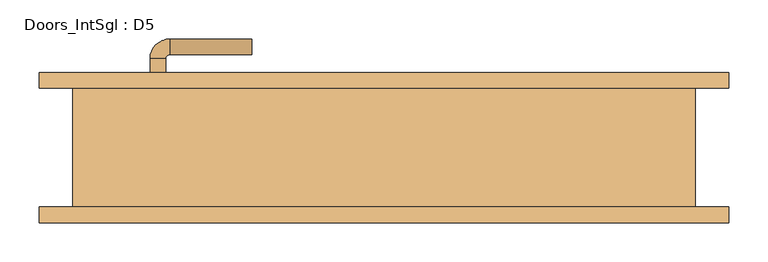
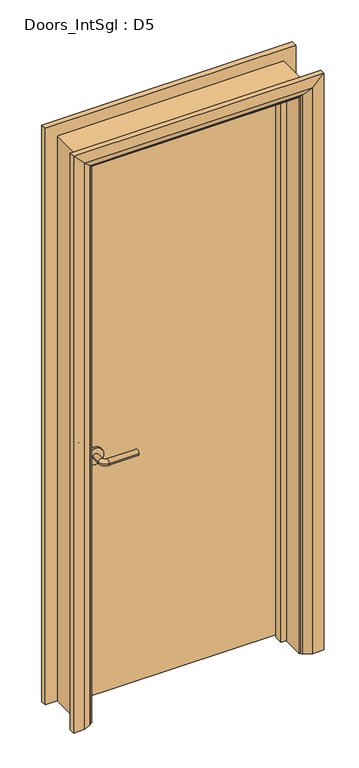
"""IFC4 building model written with IfcOpenShell, lengths in millimetres: door geometry, Doors_IntSgl : D5."""

from ifc_helpers import new_model, si_unit, point, frame, frame_2d, origin, place, context, project, spatial, polyline, circle_curve, ellipse_curve, trimmed, segment, composite_curve, outline, extrude, faceted_brep, source, transform, mapped, element, save
from ifc_brep_helpers import plane_surface, cylinder_surface, revolved_surface, advanced_brep


def doors_intsgl_d5_996c1a6b(model_context):
    return source(origin(), model_context, "Body", "SolidModel", [
        advanced_brep(
        [(-299.4508, 30.2, 900.0), (-279.4508, 30.2, 900.0), (-279.4508, 0.2, 900.0), (-299.4508, 0.2, 900.0), (-274.4508, -4.8, 900.0), (-274.4508, -24.8, 900.0), (-169.4508, -24.8, 900.0), (-169.4508, -4.8, 900.0)],
        [
            (0, 1, circle_curve(frame((-289.4508, 30.2, 900.0), z_axis=(0.0, 1.0, 0.0), x_axis=(1.0, 0.0, 0.0)), 10.0)),
            (1, 0, circle_curve(frame((-289.4508, 30.2, 900.0), z_axis=(0.0, 1.0, 0.0), x_axis=(1.0, 0.0, 0.0)), 10.0)),
            (1, 2),
            (2, 3, circle_curve(frame((-289.4508, 0.2, 900.0), z_axis=(0.0, 1.0, 0.0), x_axis=(1.0, 0.0, 0.0)), 10.0)),
            (3, 0),
            (3, 2, circle_curve(frame((-289.4508, 0.2, 900.0), z_axis=(0.0, 1.0, 0.0), x_axis=(1.0, 0.0, 0.0)), 10.0)),
            (4, 5, circle_curve(frame((-274.4508, -14.8, 900.0), z_axis=(-1.0, 0.0, 0.0), x_axis=(0.0, 1.0, 0.0)), 10.0)),
            (5, 3, circle_curve(frame((-274.4508, 0.2, 900.0), z_axis=(0.0, 0.0, -1.0), x_axis=(-1.0, 0.0, 0.0)), 25.0)),
            (2, 4, circle_curve(frame((-274.4508, 0.2, 900.0), z_axis=(0.0, 0.0, 1.0), x_axis=(-1.0, 0.0, 0.0)), 5.0)),
            (5, 4, circle_curve(frame((-274.4508, -14.8, 900.0), z_axis=(-1.0, 0.0, 0.0), x_axis=(0.0, 1.0, 0.0)), 10.0)),
            (6, 7, circle_curve(frame((-169.4508, -14.8, 900.0), z_axis=(1.0, 0.0, 0.0), x_axis=(0.0, 1.0, 0.0)), 10.0)),
            (7, 6, circle_curve(frame((-169.4508, -14.8, 900.0), z_axis=(1.0, 0.0, 0.0), x_axis=(0.0, 1.0, 0.0)), 10.0)),
            (4, 7),
            (6, 5),
        ],
        [
            plane_surface(frame((-289.4508, 30.2, 900.0), z_axis=(0.0, 1.0, 0.0), x_axis=(0.0, 0.0, 1.0))),
            cylinder_surface(frame((-289.4508, 30.2, 900.0), z_axis=(0.0, 1.0, 0.0), x_axis=(1.0, 0.0, 0.0)), 10.0),
            revolved_surface(trimmed(ellipse_curve(frame((-289.4508, 0.2, 900.0), z_axis=(0.0, -1.0, 0.0), x_axis=(1.0, 0.0, 0.0)), 10.0, 10.0), [point((-299.4508, 0.2, 900.0))], [point((-279.4508, 0.2, 900.0))], True, "CARTESIAN"), (-274.4508, 0.2, 900.0), (0.0, 0.0, -1.0)),
            revolved_surface(trimmed(ellipse_curve(frame((-289.4508, 0.2, 900.0), z_axis=(0.0, -1.0, 0.0), x_axis=(1.0, 0.0, 0.0)), 10.0, 10.0), [point((-279.4508, 0.2, 900.0))], [point((-299.4508, 0.2, 900.0))], True, "CARTESIAN"), (-274.4508, 0.2, 900.0), (0.0, 0.0, -1.0)),
            plane_surface(frame((-169.4508, -14.8, 900.0), z_axis=(1.0, 0.0, 0.0), x_axis=(0.0, 0.0, 1.0))),
            cylinder_surface(frame((-274.4508, -14.8, 900.0), z_axis=(-1.0, 0.0, 0.0), x_axis=(0.0, 1.0, 0.0)), 10.0),
        ],
        [
            (0, [[1, 2]]),
            (1, [[3, 4, 5, -2]]),
            (1, [[-5, 6, -3, -1]]),
            (2, [[7, 8, -4, 9]]),
            (3, [[10, -9, -6, -8]]),
            (4, [[11, 12]]),
            (5, [[13, -11, 14, -7]]),
            (5, [[-14, -12, -13, -10]]),
        ],
    ),
        extrude(outline(composite_curve([segment(trimmed(circle_curve(frame_2d((900.0, -291.9508)), 30.0), [point((900.0, -321.9508))], [point((900.0, -261.9508))], False, "CARTESIAN"), True, "CONTINUOUS"), segment(trimmed(circle_curve(frame_2d((900.0, -291.9508)), 30.0), [point((900.0, -261.9508))], [point((900.0, -321.9508))], False, "CARTESIAN"), True, "CONTINUOUS")], self_intersect=False)), frame((0.0, 30.2, 0.0), z_axis=(0.0, 1.0, 0.0), x_axis=(0.0, 0.0, 1.0)), (0.0, 0.0, 1.0), 8.0),
        advanced_brep(
        [(-299.4508, 84.2, 900.0), (-279.4508, 84.2, 900.0), (-299.4508, 114.2, 900.0), (-279.4508, 114.2, 900.0), (-274.4508, 119.2, 900.0), (-274.4508, 139.2, 900.0), (-169.4508, 139.2, 900.0), (-169.4508, 119.2, 900.0)],
        [
            (0, 1, circle_curve(frame((-289.4508, 84.2, 900.0), z_axis=(0.0, -1.0, 0.0), x_axis=(1.0, 0.0, 0.0)), 10.0)),
            (1, 0, circle_curve(frame((-289.4508, 84.2, 900.0), z_axis=(0.0, -1.0, 0.0), x_axis=(1.0, 0.0, 0.0)), 10.0)),
            (0, 2),
            (2, 3, circle_curve(frame((-289.4508, 114.2, 900.0), z_axis=(0.0, -1.0, 0.0), x_axis=(1.0, 0.0, 0.0)), 10.0)),
            (3, 1),
            (3, 2, circle_curve(frame((-289.4508, 114.2, 900.0), z_axis=(0.0, -1.0, 0.0), x_axis=(1.0, 0.0, 0.0)), 10.0)),
            (4, 3, circle_curve(frame((-274.4508, 114.2, 900.0), z_axis=(0.0, 0.0, 1.0), x_axis=(-1.0, 0.0, 0.0)), 5.0)),
            (2, 5, circle_curve(frame((-274.4508, 114.2, 900.0), z_axis=(0.0, 0.0, -1.0), x_axis=(-1.0, 0.0, 0.0)), 25.0)),
            (5, 4, circle_curve(frame((-274.4508, 129.2, 900.0), z_axis=(-1.0, 0.0, 0.0), x_axis=(0.0, -1.0, 0.0)), 10.0)),
            (4, 5, circle_curve(frame((-274.4508, 129.2, 900.0), z_axis=(-1.0, 0.0, 0.0), x_axis=(0.0, -1.0, 0.0)), 10.0)),
            (6, 7, circle_curve(frame((-169.4508, 129.2, 900.0), z_axis=(1.0, 0.0, 0.0), x_axis=(0.0, -1.0, 0.0)), 10.0)),
            (7, 6, circle_curve(frame((-169.4508, 129.2, 900.0), z_axis=(1.0, 0.0, 0.0), x_axis=(0.0, -1.0, 0.0)), 10.0)),
            (5, 6),
            (7, 4),
        ],
        [
            plane_surface(frame((-289.4508, 84.2, 900.0), z_axis=(0.0, -1.0, 0.0), x_axis=(0.0, 0.0, 1.0))),
            cylinder_surface(frame((-289.4508, 84.2, 900.0), z_axis=(0.0, -1.0, 0.0), x_axis=(1.0, 0.0, 0.0)), 10.0),
            revolved_surface(trimmed(ellipse_curve(frame((-289.4508, 114.2, 900.0), z_axis=(0.0, -1.0, 0.0), x_axis=(1.0, 0.0, 0.0)), 10.0, 10.0), [point((-299.4508, 114.2, 900.0))], [point((-279.4508, 114.2, 900.0))], True, "CARTESIAN"), (-274.4508, 114.2, 900.0), (0.0, 0.0, -1.0)),
            revolved_surface(trimmed(ellipse_curve(frame((-289.4508, 114.2, 900.0), z_axis=(0.0, -1.0, 0.0), x_axis=(1.0, 0.0, 0.0)), 10.0, 10.0), [point((-279.4508, 114.2, 900.0))], [point((-299.4508, 114.2, 900.0))], True, "CARTESIAN"), (-274.4508, 114.2, 900.0), (0.0, 0.0, -1.0)),
            plane_surface(frame((-169.4508, 129.2, 900.0), z_axis=(1.0, 0.0, 0.0), x_axis=(0.0, 0.0, 1.0))),
            cylinder_surface(frame((-274.4508, 129.2, 900.0), z_axis=(-1.0, 0.0, 0.0), x_axis=(0.0, -1.0, 0.0)), 10.0),
        ],
        [
            (0, [[1, 2]]),
            (1, [[-1, 3, 4, 5]]),
            (1, [[-2, -5, 6, -3]]),
            (2, [[7, -4, 8, 9]]),
            (3, [[-8, -6, -7, 10]]),
            (4, [[11, 12]]),
            (5, [[-9, 13, -12, 14]]),
            (5, [[-10, -14, -11, -13]]),
        ],
    ),
        extrude(outline(composite_curve([segment(trimmed(circle_curve(frame_2d((900.0, -291.9508)), 30.0), [point((900.0, -321.9508))], [point((900.0, -261.9508))], False, "CARTESIAN"), True, "CONTINUOUS"), segment(trimmed(circle_curve(frame_2d((900.0, -291.9508)), 30.0), [point((900.0, -261.9508))], [point((900.0, -321.9508))], False, "CARTESIAN"), True, "CONTINUOUS")], self_intersect=False)), frame((0.0, 76.2, 0.0), z_axis=(0.0, 1.0, 0.0), x_axis=(0.0, 0.0, 1.0)), (0.0, 0.0, 1.0), 8.0),
        extrude(outline(polyline([(364.4508, 38.2), (-364.4508, 38.2), (-364.4508, 76.2), (364.4508, 76.2), (364.4508, 38.2)])), frame((0.0, 0.0, 8.0), z_axis=(0.0, 0.0, 1.0), x_axis=(1.0, 0.0, 0.0)), (0.0, 0.0, 1.0), 2060.0),
        advanced_brep(
        [(441.4508, 96.2, 0.0), (441.4508, 76.2, 0.0), (371.4508, 76.2, 0.0), (375.4508, 82.2, 0.0), (401.4508, 96.2, 0.0), (441.4508, 96.2, 2145.0), (441.4508, 76.2, 2145.0), (-441.4508, 76.2, 2145.0), (-441.4508, 76.2, 0.0), (-371.4508, 76.2, 0.0), (-371.4508, 76.2, 2075.0), (371.4508, 76.2, 2075.0), (375.4508, 82.2, 2079.0), (401.4508, 96.2, 2105.0), (-401.4508, 96.2, 2105.0), (-401.4508, 96.2, 0.0), (-441.4508, 96.2, 0.0), (-441.4508, 96.2, 2145.0), (-375.4508, 82.2, 0.0), (-375.4508, 82.2, 2079.0)],
        [
            (0, 1),
            (1, 2),
            (2, 3, circle_curve(frame((379.4508, 75.2, 0.0), z_axis=(0.0, 0.0, -1.0), x_axis=(1.0, 0.0, 0.0)), 8.0622577)),
            (3, 4),
            (4, 0),
            (0, 5),
            (5, 6),
            (6, 1),
            (6, 7),
            (7, 8),
            (8, 9),
            (9, 10),
            (10, 11),
            (11, 2),
            (11, 12, ellipse_curve(frame((379.4508, 75.2, 2083.0), z_axis=(0.7071067811865475, 0.0, -0.7071067811865475), x_axis=(-0.7071067811865474, 0.0, -0.7071067811865476)), 11.4017543, 8.0622577)),
            (12, 3),
            (12, 13),
            (13, 4),
            (13, 14),
            (14, 15),
            (15, 16),
            (16, 17),
            (17, 5),
            (7, 17),
            (16, 8),
            (15, 18),
            (18, 9, circle_curve(frame((-379.4508, 75.2, 0.0), z_axis=(0.0, 0.0, -1.0), x_axis=(-1.0, 0.0, 0.0)), 8.0622577)),
            (19, 10, ellipse_curve(frame((-379.4508, 75.2, 2083.0), z_axis=(-0.7071067811865475, 0.0, -0.7071067811865475), x_axis=(-0.7071067811865474, 0.0, 0.7071067811865476)), 11.4017543, 8.0622577)),
            (18, 19),
            (14, 19),
            (19, 12),
        ],
        [
            plane_surface(frame((371.4508, 76.2, 0.0), z_axis=(0.0, 0.0, -1.0), x_axis=(0.0, -1.0, 0.0))),
            plane_surface(frame((441.4508, 96.2, 0.0), z_axis=(1.0, 0.0, 0.0), x_axis=(0.0, 0.0, 1.0))),
            plane_surface(frame((441.4508, 76.2, 0.0), z_axis=(0.0, -1.0, 0.0), x_axis=(0.0, 0.0, 1.0))),
            cylinder_surface(frame((379.4508, 75.2, 0.0), z_axis=(0.0, 0.0, -1.0), x_axis=(1.0, 0.0, 0.0)), 8.0622577),
            plane_surface(frame((375.4508, 82.2, 0.0), z_axis=(-0.4740998230350126, 0.880471099922178, 0.0), x_axis=(0.0, 0.0, 1.0))),
            plane_surface(frame((401.4508, 96.2, 0.0), z_axis=(0.0, 1.0, 0.0), x_axis=(0.0, 0.0, 1.0))),
            plane_surface(frame((-441.4508, 96.2, 2145.0), z_axis=(-1.0, 0.0, 0.0), x_axis=(0.0, 0.0, -1.0))),
            plane_surface(frame((-371.4508, 76.2, 0.0), z_axis=(0.0, 0.0, -1.0), x_axis=(0.0, -1.0, 0.0))),
            cylinder_surface(frame((-379.4508, 75.2, 2075.0), z_axis=(0.0, 0.0, 1.0), x_axis=(-1.0, 0.0, 0.0)), 8.0622577),
            plane_surface(frame((-375.4508, 82.2, 2079.0), z_axis=(0.47409982303501824, 0.8804710999221749, 0.0), x_axis=(0.0, 0.0, -1.0))),
            plane_surface(frame((441.4508, 96.2, 2145.0), z_axis=(0.0, 0.0, 1.0), x_axis=(-1.0, 0.0, 0.0))),
            cylinder_surface(frame((371.4508, 75.2, 2083.0), z_axis=(1.0, 0.0, 0.0), x_axis=(0.0, 0.0, 1.0)), 8.0622577),
            plane_surface(frame((375.4508, 82.2, 2079.0), z_axis=(0.0, 0.8804710999221764, -0.4740998230350154), x_axis=(-1.0, 0.0, 0.0))),
        ],
        [
            (0, [[1, 2, 3, 4, 5]]),
            (1, [[-1, 6, 7, 8]]),
            (2, [[-2, -8, 9, 10, 11, 12, 13, 14]]),
            (3, [[-3, -14, 15, 16]]),
            (4, [[-4, -16, 17, 18]]),
            (5, [[-5, -18, 19, 20, 21, 22, 23, -6]]),
            (6, [[24, -22, 25, -10]]),
            (7, [[-21, 26, 27, -11, -25]]),
            (8, [[28, -12, -27, 29]]),
            (9, [[30, -29, -26, -20]]),
            (10, [[-7, -23, -24, -9]]),
            (11, [[-15, -13, -28, 31]]),
            (12, [[-17, -31, -30, -19]]),
        ],
    ),
        extrude(outline(polyline([(0.0, -366.4508), (0.0, -347.4508), (2051.0, -347.4508), (2051.0, 347.4508), (0.0, 347.4508), (0.0, 366.4508), (2070.0, 366.4508), (2070.0, -366.4508), (0.0, -366.4508)])), frame((0.0, 4.2, 0.0), z_axis=(0.0, 1.0, 0.0), x_axis=(0.0, 0.0, 1.0)), (0.0, 0.0, 1.0), 32.0),
        advanced_brep(
        [(-441.4508, -96.2, 0.0), (-441.4508, -76.2, 0.0), (-371.4508, -76.2, 0.0), (-375.4508, -82.2, 0.0), (-401.4508, -96.2, 0.0), (-441.4508, -96.2, 2145.0), (-441.4508, -76.2, 2145.0), (-371.4508, -76.2, 2075.0), (-375.4508, -82.2, 2079.0), (-401.4508, -96.2, 2105.0), (441.4508, -96.2, 0.0), (401.4508, -96.2, 0.0), (375.4508, -82.2, 0.0), (371.4508, -76.2, 0.0), (441.4508, -76.2, 0.0), (441.4508, -96.2, 2145.0), (401.4508, -96.2, 2105.0), (375.4508, -82.2, 2079.0), (371.4508, -76.2, 2075.0), (441.4508, -76.2, 2145.0)],
        [
            (0, 1),
            (1, 2),
            (2, 3, circle_curve(frame((-379.4508, -75.2, 0.0), z_axis=(0.0, 0.0, -1.0), x_axis=(-1.0, 0.0, 0.0)), 8.0622577)),
            (3, 4),
            (4, 0),
            (0, 5),
            (5, 6),
            (6, 1),
            (6, 7),
            (7, 2),
            (7, 8, ellipse_curve(frame((-379.4508, -75.2, 2083.0), z_axis=(-0.7071067811865475, 0.0, -0.7071067811865475), x_axis=(0.7071067811865474, 0.0, -0.7071067811865476)), 11.4017543, 8.0622577)),
            (8, 3),
            (8, 9),
            (9, 4),
            (9, 5),
            (10, 11),
            (11, 12),
            (12, 13, circle_curve(frame((379.4508, -75.2, 0.0), z_axis=(0.0, 0.0, -1.0), x_axis=(1.0, 0.0, 0.0)), 8.0622577)),
            (13, 14),
            (14, 10),
            (15, 16),
            (16, 11),
            (10, 15),
            (16, 17),
            (17, 12),
            (17, 18, ellipse_curve(frame((379.4508, -75.2, 2083.0), z_axis=(0.7071067811865475, 0.0, -0.7071067811865475), x_axis=(0.7071067811865474, 0.0, 0.7071067811865476)), 11.4017543, 8.0622577)),
            (18, 13),
            (18, 19),
            (19, 14),
            (19, 15),
            (5, 15),
            (19, 6),
            (18, 7),
            (17, 8),
            (16, 9),
        ],
        [
            plane_surface(frame((-371.4508, -149.0010989, 0.0), z_axis=(0.0, 0.0, -1.0), x_axis=(1.0, 0.0, 0.0))),
            plane_surface(frame((-441.4508, -96.2, 0.0), z_axis=(-1.0, 0.0, 0.0), x_axis=(0.0, 0.0, 1.0))),
            plane_surface(frame((-441.4508, -76.2, 0.0), z_axis=(0.0, 1.0, 0.0), x_axis=(0.0, 0.0, 1.0))),
            cylinder_surface(frame((-379.4508, -75.2, 0.0), z_axis=(0.0, 0.0, -1.0), x_axis=(-1.0, 0.0, 0.0)), 8.0622577),
            plane_surface(frame((-375.4508, -82.2, 0.0), z_axis=(0.4740998230350183, -0.8804710999221749, 0.0), x_axis=(0.0, 0.0, 1.0))),
            plane_surface(frame((-401.4508, -96.2, 0.0), z_axis=(0.0, -1.0, 0.0), x_axis=(0.0, 0.0, 1.0))),
            plane_surface(frame((371.4508, -149.0010989, 0.0), z_axis=(0.0, 0.0, -1.0), x_axis=(-1.0, 0.0, 0.0))),
            plane_surface(frame((401.4508, -96.2, 2105.0), z_axis=(0.0, -1.0, 0.0), x_axis=(0.0, 0.0, -1.0))),
            plane_surface(frame((375.4508, -82.2, 2079.0), z_axis=(-0.4740998230350183, -0.8804710999221749, 0.0), x_axis=(0.0, 0.0, -1.0))),
            cylinder_surface(frame((379.4508, -75.2, 2075.0), z_axis=(0.0, 0.0, 1.0), x_axis=(1.0, 0.0, 0.0)), 8.0622577),
            plane_surface(frame((441.4508, -76.2, 2145.0), z_axis=(0.0, 1.0, 0.0), x_axis=(0.0, 0.0, -1.0))),
            plane_surface(frame((441.4508, -96.2, 2145.0), z_axis=(1.0, 0.0, 0.0), x_axis=(0.0, 0.0, -1.0))),
            plane_surface(frame((-441.4508, -96.2, 2145.0), z_axis=(0.0, 0.0, 1.0), x_axis=(1.0, 0.0, 0.0))),
            plane_surface(frame((-441.4508, -76.2, 2145.0), z_axis=(0.0, 1.0, 0.0), x_axis=(1.0, 0.0, 0.0))),
            cylinder_surface(frame((-371.4508, -75.2, 2083.0), z_axis=(-1.0, 0.0, 0.0), x_axis=(0.0, 0.0, 1.0)), 8.0622577),
            plane_surface(frame((-375.4508, -82.2, 2079.0), z_axis=(0.0, -0.8804710999221749, -0.4740998230350183), x_axis=(1.0, 0.0, 0.0))),
            plane_surface(frame((-401.4508, -96.2, 2105.0), z_axis=(0.0, -1.0, 0.0), x_axis=(1.0, 0.0, 0.0))),
        ],
        [
            (0, [[1, 2, 3, 4, 5]]),
            (1, [[-1, 6, 7, 8]]),
            (2, [[-2, -8, 9, 10]]),
            (3, [[-3, -10, 11, 12]]),
            (4, [[-4, -12, 13, 14]]),
            (5, [[-5, -14, 15, -6]]),
            (6, [[16, 17, 18, 19, 20]]),
            (7, [[21, 22, -16, 23]]),
            (8, [[24, 25, -17, -22]]),
            (9, [[26, 27, -18, -25]]),
            (10, [[28, 29, -19, -27]]),
            (11, [[30, -23, -20, -29]]),
            (12, [[-7, 31, -30, 32]]),
            (13, [[-9, -32, -28, 33]]),
            (14, [[-11, -33, -26, 34]]),
            (15, [[-13, -34, -24, 35]]),
            (16, [[-15, -35, -21, -31]]),
        ],
    ),
        faceted_brep([(-366.4508, 76.2, 0.0), (-366.4508, -76.2, 0.0), (-398.4508, -76.2, 0.0), (-398.4508, 76.2, 0.0), (-366.4508, 76.2, 2070.0), (-366.4508, -76.2, 2070.0), (-398.4508, -76.2, 2102.0), (-398.4508, 76.2, 2102.0), (366.4508, 76.2, 0.0), (398.4508, 76.2, 0.0), (398.4508, -76.2, 0.0), (366.4508, -76.2, 0.0), (366.4508, 76.2, 2070.0), (398.4508, 76.2, 2102.0), (398.4508, -76.2, 2102.0), (366.4508, -76.2, 2070.0)], [[[0, 1, 2, 3]], [[1, 0, 4, 5]], [[2, 1, 5, 6]], [[3, 2, 6, 7]], [[0, 3, 7, 4]], [[8, 9, 10, 11]], [[12, 13, 9, 8]], [[13, 14, 10, 9]], [[14, 15, 11, 10]], [[15, 12, 8, 11]], [[5, 4, 12, 15]], [[6, 5, 15, 14]], [[7, 6, 14, 13]], [[4, 7, 13, 12]]]),
    ])


if __name__ == "__main__":
    model = new_model("IFC4")
    model_context = context("Model", 3, world=origin())
    ifc_project = project(units=[si_unit("LENGTHUNIT", "METRE", prefix="MILLI")], contexts=[model_context])
    site = spatial("IfcSite", under=ifc_project)
    building = spatial("IfcBuilding", under=site)
    placement = place(None, origin())
    doors_intsgl_d5_shape = doors_intsgl_d5_996c1a6b(model_context)
    element("IfcDoor", 1, ObjectType="Doors_IntSgl : D5", at=placement, inside=building, context=model_context, shape_type="MappedRepresentation", body=[
        mapped(doors_intsgl_d5_shape, transform((0.0, 0.0, 0.0), x_axis=(1.0, 0.0, 0.0), y_axis=(0.0, 1.0, 0.0), z_axis=(0.0, 0.0, 1.0))),
    ])
    save(model, "model.ifc")

# Revit data of these elements
# Type "Doors_IntSgl : D5"
#   Type Mark = "48"
#   Type Comments = "Internal Single"
#   Operation = "SingleSwingRight"
#   Manufacturer = "Revit"
#   Keynote = "L20"
#   Description = "Internal Single Door"
#   Analytic Construction = "Metal"
#   UnderCut = 0.026247 ft
#   Tolerance = 0.006562 ft
#   Thickness = 0.124672 ft
#   Thermal Resistance (R) = 0.270117 (m²·K)/W
#   Structural Tolerance = 0.026247 ft
#   StopDepth = 0.104987 ft
#   Stop Thickness = 0.062336 ft
#   Rough Width = 2.667 ft
#   Rough Height = 6.922572 ft
#   Height to Top Lock Rail = 3.28084 ft
#   Heat Transfer Coefficient (U) = 3.7021 W/(m²·K)
#   Handle Z Distance = 2.952756 ft
#   Handle X Distance = 0.246063 ft
#   Frame Thickness = 0.104987 ft
#   Door Panel Width = 2.391409 ft
#   Door Panel Thickness = 0.124672 ft
#   Door Panel Offset = 0.0 ft
#   Height = 6.922572 ft
#   Width = 2.667 ft
#   Door Panel Height = 6.75853 ft
#   Architrave Setback = 0.016404 ft
#   Vis - Ironmongery = yes
#   Material Ironmongery = Door - Handle
#   Material Frame = Door - Frame/Mullion (1)
#   Material Door = Door - Panel
#   Material Architrave = Door - Architrave
#   Visual Light Transmittance = 0
#   Solar Heat Gain Coefficient = 0
#   Function = (empty or 0)
#   Wall Closure = (empty or 0)
# Element 1 (IfcDoor, "Doors_IntSgl : D5")
#   Materials on its faces: "Door - Architrave", "Door - Handle", "Door - Frame/Mullion (1)", "Door - Panel"
# Materials
#   "Door - Handle": colour RGB 0 0 0, transparency 0, Keynote = "P21", Cost = 0
#   "Door - Frame/Mullion (1)": class "Wood", colour RGB 212 179 113, transparency 0, Keynote = "L20", Cost = 0
#   "Door - Panel": class "Wood", colour RGB 210 159 95, transparency 0, Keynote = "L20", Cost = 0
#   "Door - Architrave": class "Wood", colour RGB 154 90 5, transparency 0, Keynote = "P20", Cost = 0
